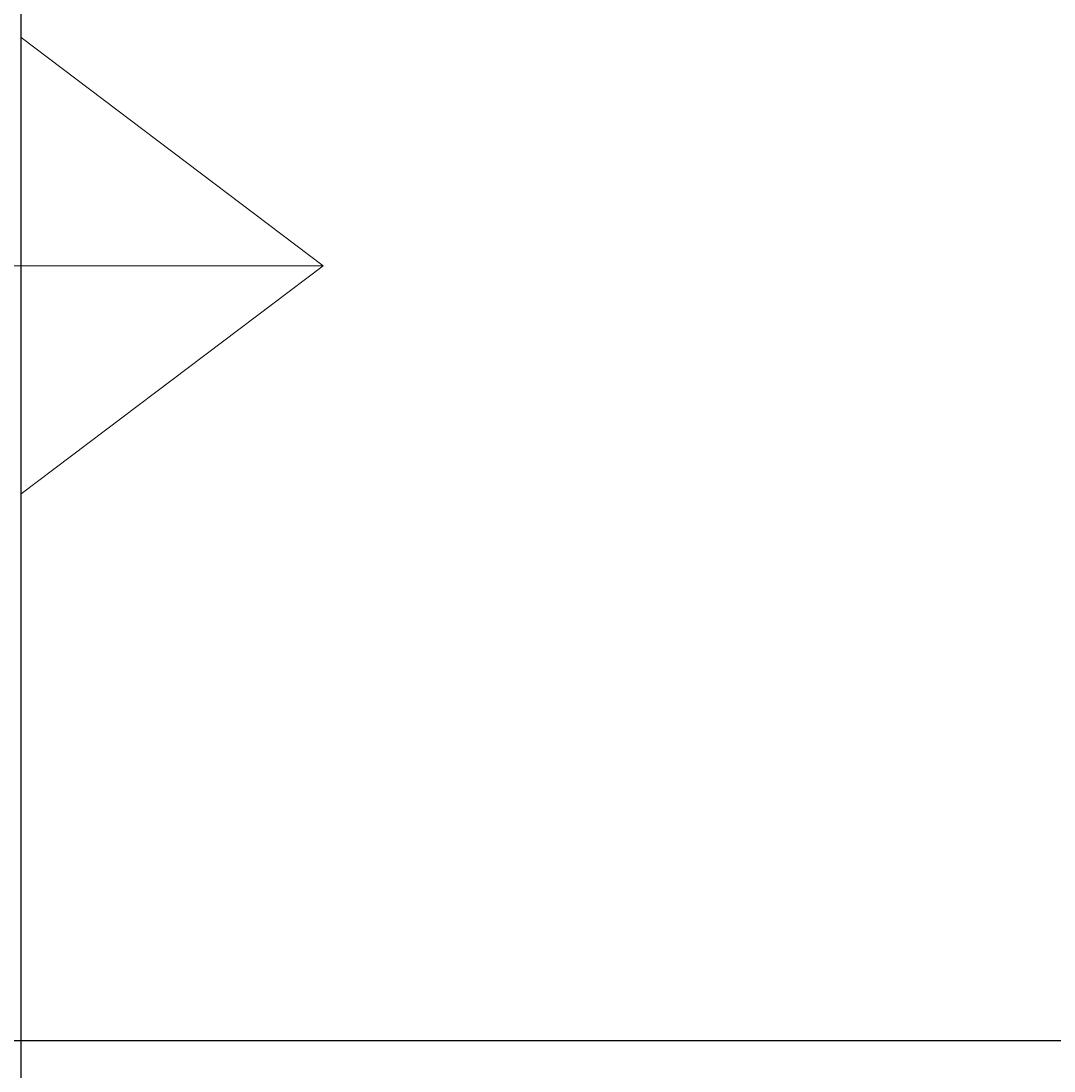
# Model space of a CAD drawing. Units: inches. Extents: x 1998 to 2588, y 1139 to 1977.
# Tile 118 of 134: x 2498 to 2524, y 1595 to 1622. Entities that reach past the tile are written whole.
import ezdxf

# ---------------------------------------------------------------- set-up
doc = ezdxf.new("R2010")
doc.units = ezdxf.units.IN
for name, color, linetype, lineweight in [('A-ANNO-DIMS', 2, 'Continuous', 18), ('A-ANNO-SYMB', 7, 'Continuous', 18), ('A-FLOR-STRS', 7, 'Continuous', 25)]:
    doc.layers.add(name, color=color, linetype=linetype, lineweight=lineweight)
doc.styles.get("Standard").update_dxf_attribs({"font": 'arial.ttf'})
doc.dimstyles.get("Standard").update_dxf_attribs({"dimtxt": 0.18, "dimasz": 0.18, "dimexe": 0.18, "dimexo": 0.0625, "dimgap": 0.09, "dimtad": 0, "dimtih": 1, "dimtoh": 1, "dimdec": 4, "dimzin": 0, "dimdsep": 46, "dimtxsty": 'Standard', "dimcen": 0.09, "dimadec": 0, "dimazin": 0, "dimtfac": 1, "dimtdec": 4, "dimtofl": 0, "dimtmove": 0, "dimatfit": 3, "dimfxl": 1, "dimtolj": 1, "dimtzin": 0, "dimarcsym": 0})

# ---------------------------------------------------------------- blocks, each defined once
blk = doc.blocks.new('*D24')
at = {"layer": 'A-ANNO-DIMS', "color": 0, "lineweight": -2, "transparency": 16777216}
for p, q in [((2398.535, 1911.232), (2588.309, 1911.232)), ((2588.129, 1911.052), (2588.129, 1570.164)), ((2588.129, 1228.912), (2588.129, 1569.8)), ((2527.535, 1228.732), (2588.309, 1228.732))]:
    blk.add_line(p, q, dxfattribs=at)
at = {"layer": 'A-ANNO-DIMS', "color": 0, "transparency": 16777216}
for points in [[(2588.099, 1911.052), (2588.159, 1911.052), (2588.129, 1911.232)], [(2588.099, 1228.912), (2588.159, 1228.912), (2588.129, 1228.732)]]:
    blk.add_solid(points, dxfattribs=at)
at = {"layer": 'Defpoints', "color": 0, "transparency": 16777216}
for p in [(2398.473, 1911.232), (2588.129, 1911.232), (2527.473, 1228.732)]:
    blk.add_point(p, dxfattribs=at)
at = {"layer": 'A-ANNO-DIMS', "color": 0, "transparency": 16777216, "insert": (2588.129, 1569.982), "char_height": 0.18, "attachment_point": 5}
blk.add_mtext('\\A1;682.5', dxfattribs=at)
blk = doc.blocks.new('*D39')
at = {"layer": 'A-ANNO-DIMS', "color": 0, "lineweight": -2, "transparency": 16777216}
for p, q in [((2115.035, 1628.742), (2588.309, 1628.742)), ((2588.129, 1628.562), (2588.129, 1612.685)), ((2588.129, 1596.444), (2588.129, 1612.321)), ((2115.035, 1596.264), (2588.309, 1596.264))]:
    blk.add_line(p, q, dxfattribs=at)
at = {"layer": 'A-ANNO-DIMS', "color": 0, "transparency": 16777216}
for points in [[(2588.099, 1628.562), (2588.159, 1628.562), (2588.129, 1628.742)], [(2588.099, 1596.444), (2588.159, 1596.444), (2588.129, 1596.264)]]:
    blk.add_solid(points, dxfattribs=at)
at = {"layer": 'Defpoints', "color": 0, "transparency": 16777216}
for p in [(2114.973, 1628.742), (2588.129, 1628.742), (2114.973, 1596.264)]:
    blk.add_point(p, dxfattribs=at)
at = {"layer": 'A-ANNO-DIMS', "color": 0, "transparency": 16777216, "insert": (2588.129, 1612.503), "char_height": 0.18, "attachment_point": 5}
blk.add_mtext('\\A1;32.48', dxfattribs=at)

msp = doc.modelspace()

# ---------------------------------------------------------------- linework, layer by layer
at = {"layer": 'A-ANNO-SYMB'}
for p, q in [((2505.7676, 1615.7324), (2498.1786, 1621.4684)), ((2407.9729, 1615.7324), (2505.7676, 1615.7324)), ((2505.7676, 1615.7324), (2498.1786, 1609.9963))]:
    msp.add_line(p, q, dxfattribs=at)
at = {"layer": 'A-FLOR-STRS'}
msp.add_line((2498.1786, 1480.7324), (2498.1786, 1636.7324), dxfattribs=at)

# ---------------------------------------------------------------- dimensions: what is measured, and where the dimension line sits
at = {"layer": 'A-ANNO-DIMS'}
for base, p1, p2, override, picture, middle in [((2588.1286, 1911.2324), (2527.4729, 1228.7324), (2398.4729, 1911.2324), {"dimdec": 1, "dimlfac": 1, "dimrnd": 0, "dimzin": 0, "dimdsep": 46, "dimlunit": 2}, '*D24', (2588.1286, 1569.9824)), ((2588.1286, 1628.7416), (2114.9729, 1596.2642), (2114.9729, 1628.7416), {"dimdec": 2, "dimlfac": 1, "dimrnd": 0, "dimzin": 0, "dimdsep": 46, "dimlunit": 2}, '*D39', (2588.1286, 1612.5029))]:
    dim = msp.add_linear_dim(base=base, p1=p1, p2=p2, angle=90, dimstyle='Standard', override=override, dxfattribs=at)
    dim.commit()
    dim.dimension.update_dxf_attribs({"geometry": picture, "text_midpoint": middle})

doc.saveas('drawing.dxf')
